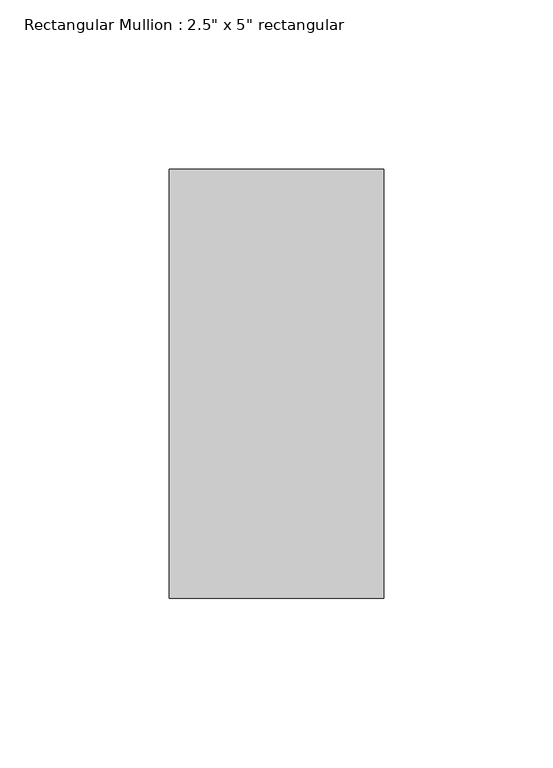
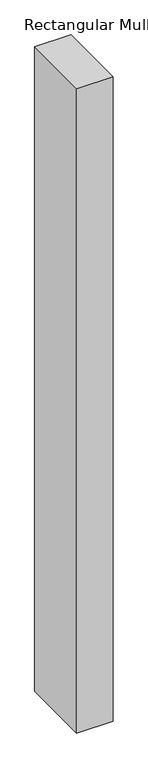
"""IFC4 building model written with IfcOpenShell, lengths in millimetres: member geometry."""

from ifc_helpers import new_model, si_unit, frame, origin, place, context, project, spatial, polyline, outline, extrude, source, transform, mapped, element, save


def member_7f33020a(model_context):
    return source(origin(), model_context, "Body", "SweptSolid", [
        extrude(outline(polyline([(0.0, 63.5), (0.0, -63.5), (-63.5, -63.5), (-63.5, 63.5), (0.0, 63.5)])), frame((0.0, 0.0, -1190.625), z_axis=(0.0, 0.0, 1.0), x_axis=(1.0, 0.0, 0.0)), (0.0, 0.0, 1.0), 1190.625),
    ])


if __name__ == "__main__":
    model = new_model("IFC4")
    model_context = context("Model", 3, world=origin())
    ifc_project = project(units=[si_unit("LENGTHUNIT", "METRE", prefix="MILLI")], contexts=[model_context])
    site = spatial("IfcSite", under=ifc_project)
    building = spatial("IfcBuilding", under=site)
    placement = place(None, origin())
    member_shape = member_7f33020a(model_context)
    element("IfcMember", 1, ObjectType="Rectangular Mullion : 2.5\" x 5\" rectangular", at=placement, inside=building, context=model_context, shape_type="MappedRepresentation", body=[
        mapped(member_shape, transform((0.0, 0.0, 0.0), x_axis=(1.0, 0.0, 0.0), y_axis=(0.0, 1.0, 0.0), z_axis=(0.0, 0.0, 1.0))),
    ])
    save(model, "model.ifc")

# Revit data of these elements
# Type "Rectangular Mullion : 2.5\" x 5\" rectangular"
#   built-in parameter 1007304 = 0.416667 (stored number, unit not read)
#   built-in parameter 1007301 = 0.104167 (stored number, unit not read)
#   built-in parameter 1007300 = 0.104167 (stored number, unit not read)
# Element 1 (IfcMember, "Rectangular Mullion : 2.5\" x 5\" rectangular")
#   Materials on its faces: "Aluminum"
# Materials
#   "Aluminum": class "Metal", colour RGB 247 247 247, transparency 0, Description = "Aluminum 6061", Cost = 0
